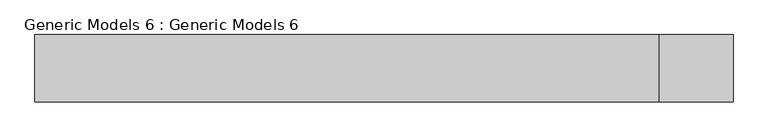
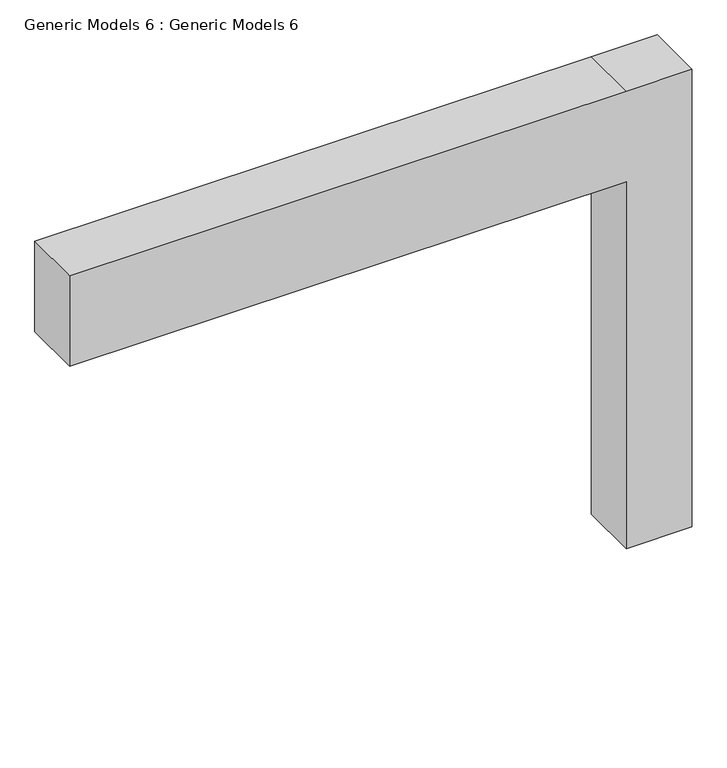
"""IFC4 building model written with IfcOpenShell, lengths in millimetres: proxy geometry, Generic Models 6 : Generic Models 6."""

from ifc_helpers import new_model, si_unit, frame, origin, place, context, project, spatial, polyline, outline, extrude, source, transform, mapped, element, save


def generic_models_6_generic_models_6_c23547c4(model_context):
    return source(origin(), model_context, "Body", "SweptSolid", [
        extrude(outline(polyline([(2535.3869158, -14425.5406521), (2535.3869158, -10564.7406521), (-152.4, -10564.7406521), (-152.4, -10107.5406521), (3200.4, -10107.5406521), (3200.4, -10564.7406521), (3200.4, -14425.5406521), (2535.3869158, -14425.5406521)])), frame((0.0, -12713.6145901, 0.0), z_axis=(0.0, 1.0, 0.0), x_axis=(0.0, 0.0, 1.0)), (0.0, 0.0, 1.0), 416.6835109),
    ])


if __name__ == "__main__":
    model = new_model("IFC4")
    model_context = context("Model", 3, world=origin())
    ifc_project = project(units=[si_unit("LENGTHUNIT", "METRE", prefix="MILLI")], contexts=[model_context])
    site = spatial("IfcSite", under=ifc_project)
    building = spatial("IfcBuilding", under=site)
    placement = place(None, origin())
    generic_models_6_generic_models_6_shape = generic_models_6_generic_models_6_c23547c4(model_context)
    element("IfcBuildingElementProxy", 1, Name="Generic Models 6 : Generic Models 6", ObjectType="Generic Models 6 : Generic Models 6", at=placement, inside=building, context=model_context, shape_type="MappedRepresentation", body=[
        mapped(generic_models_6_generic_models_6_shape, transform((0.0, 0.0, 0.0), x_axis=(1.0, 0.0, 0.0), y_axis=(0.0, 1.0, 0.0), z_axis=(0.0, 0.0, 1.0))),
    ])
    save(model, "model.ifc")

# Revit data of these elements
# Element 1 (IfcBuildingElementProxy, "Generic Models 6 : Generic Models 6")
#   Materials on its faces: "GREY COLOUR FRAME(2)"
# Materials
#   "GREY COLOUR FRAME(2)": class "Generic", colour RGB 120 120 120, transparency 0, Cost = 0
